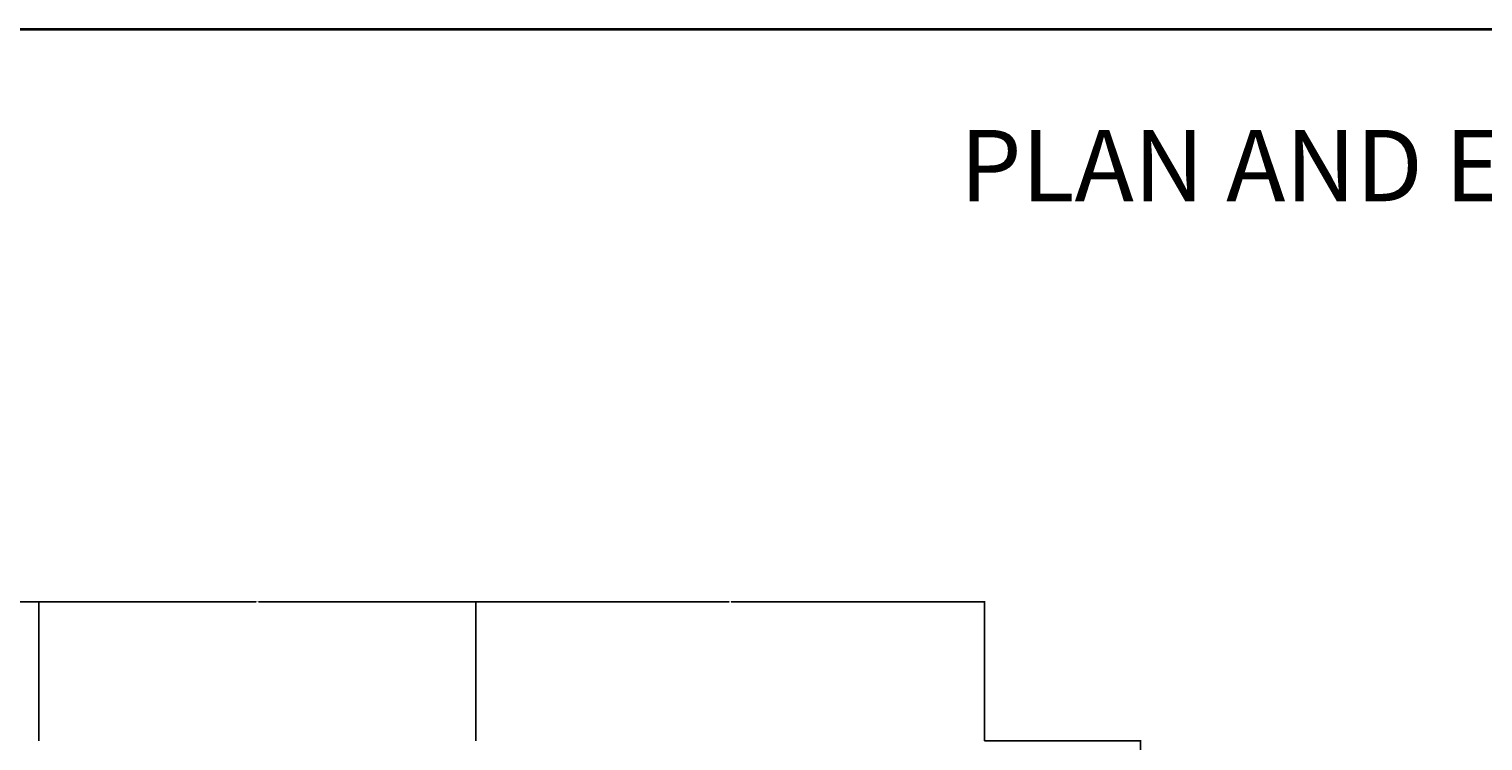
# Model space of a CAD drawing. Units: inches. Extents: x 2220 to 3422, y 783 to 1748.
# Tile 6 of 7: x 2475 to 2821, y 1578 to 1748. Entities that reach past the tile are written whole.
import ezdxf

# ---------------------------------------------------------------- set-up
doc = ezdxf.new("R2010")
doc.units = ezdxf.units.IN
for name, color, linetype, lineweight in [('A-ANNO-DIMS', 2, 'Continuous', 18), ('A-ANNO-TEXT', 7, 'Continuous', 30), ('A-ANNO-TTLB', 7, 'Continuous', 35)]:
    doc.layers.add(name, color=color, linetype=linetype, lineweight=lineweight)
doc.styles.get("Standard").update_dxf_attribs({"font": 'arial.ttf'})
doc.dimstyles.get("Standard").update_dxf_attribs({"dimtxt": 0.18, "dimasz": 0.18, "dimexe": 0.18, "dimexo": 0.0625, "dimgap": 0.09, "dimtad": 0, "dimtih": 1, "dimtoh": 1, "dimdec": 4, "dimzin": 0, "dimdsep": 46, "dimtxsty": 'Standard', "dimcen": 0.09, "dimadec": 0, "dimazin": 0, "dimtfac": 1, "dimtdec": 4, "dimtofl": 0, "dimtmove": 0, "dimatfit": 3, "dimfxl": 1, "dimtolj": 1, "dimtzin": 0, "dimarcsym": 0})

# ---------------------------------------------------------------- blocks, each defined once
blk = doc.blocks.new('*D56')
at = {"layer": 'A-ANNO-DIMS', "color": 0, "lineweight": -2, "transparency": 16777216}
for p, q in [((2702.61, 1578.39), (2739.88, 1578.39)), ((2739.7, 1578.21), (2739.7, 1438.07)), ((2739.7, 1297.57), (2739.7, 1437.71)), ((2702.61, 1297.39), (2739.88, 1297.39))]:
    blk.add_line(p, q, dxfattribs=at)
at = {"layer": 'A-ANNO-DIMS', "color": 0, "transparency": 16777216}
for points in [[(2739.67, 1578.21), (2739.73, 1578.21), (2739.7, 1578.39)], [(2739.67, 1297.57), (2739.73, 1297.57), (2739.7, 1297.39)]]:
    blk.add_solid(points, dxfattribs=at)
at = {"layer": 'Defpoints', "color": 0, "transparency": 16777216}
for p in [(2702.55, 1578.39), (2739.7, 1578.39), (2702.55, 1297.39)]:
    blk.add_point(p, dxfattribs=at)
at = {"layer": 'A-ANNO-DIMS', "color": 0, "transparency": 16777216, "insert": (2739.7, 1437.89), "char_height": 0.18, "attachment_point": 5}
blk.add_mtext('\\A1;281', dxfattribs=at)
blk = doc.blocks.new('*D58')
at = {"layer": 'A-ANNO-DIMS', "color": 0, "lineweight": -2, "transparency": 16777216}
for p, q in [((2276.05, 1578.45), (2276.05, 1611.72)), ((2276.23, 1611.54), (2376.4, 1611.54)), ((2477.37, 1611.54), (2377.19, 1611.54)), ((2477.55, 1578.45), (2477.55, 1611.72))]:
    blk.add_line(p, q, dxfattribs=at)
at = {"layer": 'A-ANNO-DIMS', "color": 0, "transparency": 16777216}
for points in [[(2276.23, 1611.57), (2276.23, 1611.51), (2276.05, 1611.54)], [(2477.37, 1611.57), (2477.37, 1611.51), (2477.55, 1611.54)]]:
    blk.add_solid(points, dxfattribs=at)
at = {"layer": 'Defpoints', "color": 0, "transparency": 16777216}
for p in [(2477.55, 1611.54), (2276.05, 1578.39), (2477.55, 1578.39)]:
    blk.add_point(p, dxfattribs=at)
at = {"layer": 'A-ANNO-DIMS', "color": 0, "transparency": 16777216, "insert": (2376.8, 1611.54), "char_height": 0.18, "attachment_point": 5}
blk.add_mtext('\\A1;201.5', dxfattribs=at)
blk = doc.blocks.new('*D59')
at = {"layer": 'A-ANNO-DIMS', "color": 0, "lineweight": -2, "transparency": 16777216}
for p, q in [((2477.55, 1578.45), (2477.55, 1611.72)), ((2477.73, 1611.54), (2529.27, 1611.54)), ((2581.37, 1611.54), (2529.83, 1611.54)), ((2581.55, 1578.45), (2581.55, 1611.72))]:
    blk.add_line(p, q, dxfattribs=at)
at = {"layer": 'A-ANNO-DIMS', "color": 0, "transparency": 16777216}
for points in [[(2477.73, 1611.57), (2477.73, 1611.51), (2477.55, 1611.54)], [(2581.37, 1611.57), (2581.37, 1611.51), (2581.55, 1611.54)]]:
    blk.add_solid(points, dxfattribs=at)
at = {"layer": 'Defpoints', "color": 0, "transparency": 16777216}
for p in [(2581.55, 1611.54), (2477.55, 1578.39), (2581.55, 1578.39)]:
    blk.add_point(p, dxfattribs=at)
at = {"layer": 'A-ANNO-DIMS', "color": 0, "transparency": 16777216, "insert": (2529.55, 1611.54), "char_height": 0.18, "attachment_point": 5}
blk.add_mtext('\\A1;104', dxfattribs=at)
blk = doc.blocks.new('*D60')
at = {"layer": 'A-ANNO-DIMS', "color": 0, "lineweight": -2, "transparency": 16777216}
for p, q in [((2581.55, 1578.45), (2581.55, 1611.72)), ((2581.73, 1611.54), (2641.78, 1611.54)), ((2702.37, 1611.54), (2642.31, 1611.54)), ((2702.55, 1578.45), (2702.55, 1611.72))]:
    blk.add_line(p, q, dxfattribs=at)
at = {"layer": 'A-ANNO-DIMS', "color": 0, "transparency": 16777216}
for points in [[(2581.73, 1611.57), (2581.73, 1611.51), (2581.55, 1611.54)], [(2702.37, 1611.57), (2702.37, 1611.51), (2702.55, 1611.54)]]:
    blk.add_solid(points, dxfattribs=at)
at = {"layer": 'Defpoints', "color": 0, "transparency": 16777216}
for p in [(2702.55, 1611.54), (2581.55, 1578.39), (2702.55, 1578.39)]:
    blk.add_point(p, dxfattribs=at)
at = {"layer": 'A-ANNO-DIMS', "color": 0, "transparency": 16777216, "insert": (2642.05, 1611.54), "char_height": 0.18, "attachment_point": 5}
blk.add_mtext('\\A1;121', dxfattribs=at)

msp = doc.modelspace()

# ---------------------------------------------------------------- linework, layer by layer
at = {"layer": 'A-ANNO-TTLB'}
msp.add_lwpolyline([(2220.0037, 1747.9465), (3422.343, 1747.9465), (3422.343, 782.804), (2220.0037, 782.804)], close=True, dxfattribs=at)

# ---------------------------------------------------------------- texts
at = {"layer": 'A-ANNO-TEXT'}
msp.add_text('PLAN AND ELEVATION', height=17, dxfattribs=at).set_placement((2696.7314, 1706.9332))

# ---------------------------------------------------------------- dimensions: what is measured, and where the dimension line sits
at = {"layer": 'A-ANNO-DIMS'}
for base, p1, p2, override, picture, middle in [((2477.5466, 1611.5407), (2276.0466, 1578.3907), (2477.5466, 1578.3907), {"dimdec": 1, "dimlfac": 1, "dimrnd": 0, "dimzin": 0, "dimdsep": 46, "dimlunit": 2}, '*D58', (2376.7966, 1611.5407)), ((2581.5466, 1611.5407), (2477.5466, 1578.3907), (2581.5466, 1578.3907), {"dimdec": 0, "dimlfac": 1, "dimrnd": 0, "dimzin": 0, "dimdsep": 46, "dimlunit": 2}, '*D59', (2529.5466, 1611.5407)), ((2702.5466, 1611.5407), (2581.5466, 1578.3907), (2702.5466, 1578.3907), {"dimdec": 0, "dimlfac": 1, "dimrnd": 0, "dimzin": 0, "dimdsep": 46, "dimlunit": 2}, '*D60', (2642.0466, 1611.5407))]:
    dim = msp.add_linear_dim(base=base, p1=p1, p2=p2, dimstyle='Standard', override=override, dxfattribs=at)
    dim.commit()
    dim.dimension.update_dxf_attribs({"geometry": picture, "text_midpoint": middle})
dim = msp.add_linear_dim(base=(2739.6966, 1578.3907), p1=(2702.5466, 1297.3907), p2=(2702.5466, 1578.3907), angle=90, dimstyle='Standard', override={"dimdec": 0, "dimlfac": 1, "dimrnd": 0, "dimzin": 0, "dimdsep": 46, "dimlunit": 2}, dxfattribs=at)
dim.commit()
dim.dimension.update_dxf_attribs({"geometry": '*D56', "text_midpoint": (2739.6966, 1437.8907)})

doc.saveas('drawing.dxf')
